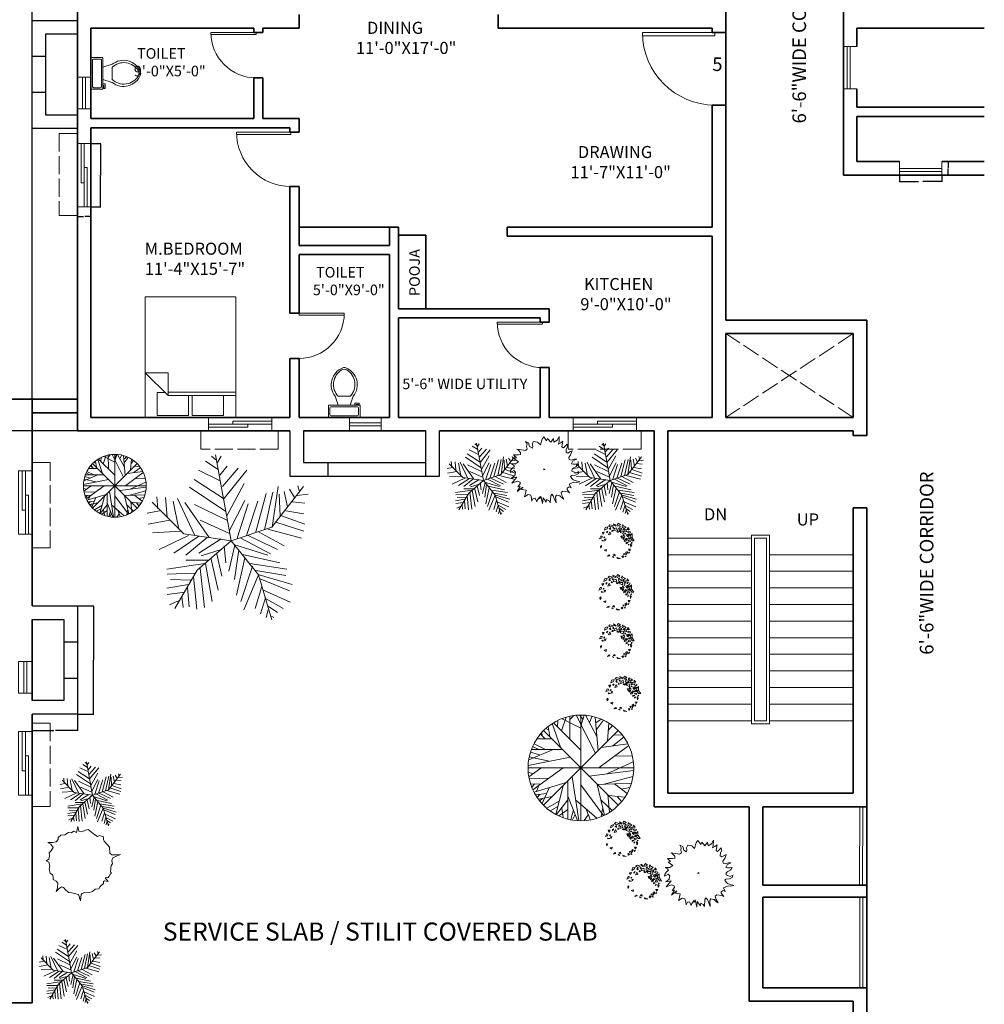
# Model space of a CAD drawing. Units: inches. Extents: x -69 to 2453, y 4803 to 7122.
# Tile 7 of 9: x 1203 to 1843, y 5759 to 6411. Entities that reach past the tile are written whole.
import ezdxf

# ---------------------------------------------------------------- set-up
doc = ezdxf.new("R2010")
doc.units = ezdxf.units.IN
doc.linetypes.add('ACAD_ISO02W100', pattern=[15, 12, -3])
for name, color, linetype, lineweight in [('A-ANNO-DIMS', 2, 'Continuous', 18), ('A-ANNO-IDEN', 2, 'Continuous', 18), ('A-ANNO-TEXT', 7, 'Continuous', 18), ('A-AREA-IDEN', 7, 'Continuous', 18), ('A-DOOR', 3, 'Continuous', 18), ('A-FLOR-FIXT', 9, 'Continuous', 18), ('A-FLOR-OPEN', 8, 'ACAD_ISO02W100', 13), ('A-FLOR-OVHD', 8, 'ACAD_ISO02W100', 13), ('A-FLOR-STRS', 4, 'Continuous', 18), ('A-FURN', 8, 'Continuous', 18), ('A-GLAZ', 244, 'Continuous', 18), ('A-WALL', 7, 'Continuous', 35), ('A-WALL-SRVC', 7, 'Continuous', 30), ('L-PLNT', 94, 'Continuous', 13)]:
    doc.layers.add(name, color=color, linetype=linetype, lineweight=lineweight)
doc.styles.get("Standard").update_dxf_attribs({"font": 'arial.ttf'})
doc.dimstyles.get("Standard").update_dxf_attribs({"dimtxt": 0.18, "dimasz": 0.18, "dimexe": 0.18, "dimexo": 0.0625, "dimgap": 0.09, "dimtad": 0, "dimtih": 1, "dimtoh": 1, "dimdec": 4, "dimzin": 0, "dimdsep": 46, "dimtxsty": 'Standard', "dimcen": 0.09, "dimadec": 0, "dimazin": 0, "dimtfac": 1, "dimtdec": 4, "dimtofl": 0, "dimtmove": 0, "dimatfit": 3, "dimfxl": 1, "dimtolj": 1, "dimtzin": 0, "dimarcsym": 0})

# ---------------------------------------------------------------- blocks, each defined once
blk = doc.blocks.new('*U9')
for p, q in [((0, 0), (0, 6)), ((40, 0), (40, 6))]:
    blk.add_line(p, q)
blk.add_lwpolyline([(0, 0), (0, -40), (1.75, -40), (1.75, 0)], close=True)
blk.add_arc((0, 0), 40, 270, 360)
blk = doc.blocks.new('*U8')
for p, q in [((0, 0), (0, 6)), ((40, 0), (40, 6))]:
    blk.add_line(p, q)
blk.add_lwpolyline([(0, 0), (0, -40), (1.75, -40), (1.75, 0)], close=True)
blk.add_arc((0, 0), 40, 270, 0)
blk = doc.blocks.new('*U5')
for p, q in [((0, 0), (0, -6)), ((40, 0), (40, -6))]:
    blk.add_line(p, q)
blk.add_lwpolyline([(0, 0), (0, 40), (1.75, 40), (1.75, 0)], close=True)
blk.add_arc((0, 0), 40, 0, 90)
blk = doc.blocks.new('*U25')
for p, q in [((-8.737, 47.138), (-17.069, 52.711)), ((-10.186, 53.64), (-13.084, 55.962)), ((0, 0), (-10.5, 57)), ((-9.099, 51.782), (-6.563, 55.962)), ((-7.288, 39.707), (-21.778, 46.673)), ((-7.65, 43.423), (-2.578, 49.46)), ((-5.839, 35.992), (4.667, 48.067)), ((-5.114, 27.632), (10.463, 46.673)), ((-5.114, 28.097), (-24.676, 40.636)), ((-3.665, 19.273), (-27.574, 35.527)), ((-2.941, 16.486), (8.652, 37.85)), ((27, 9), (48, 36)), ((27.127, 9.056), (31.112, 35.992)), ((35.096, 32.741), (37.27, 22.524)), ((38.719, 34.134), (41.979, 28.561)), ((44.153, 36.456), (45.239, 32.741)), ((-48.585, 21.131), (-49.309, 29.026)), ((-43.513, 28.561), (-42.427, 15.558)), ((-38.442, 26.239), (-34.819, 7.663)), ((-35.544, 28.097), (-24.314, 3.947)), ((-1.129, 6.734), (9.014, 26.704)), ((10.101, 3.483), (17.708, 26.239)), ((16.259, 5.805), (23.142, 31.348)), ((22.055, 7.198), (27.489, 32.277)), ((31.836, 30.883), (32.561, 16.486)), ((43.791, 29.954), (51.036, 30.883)), ((-47.498, 19.737), (-55.83, 18.344)), ((-31.5, 4.5), (-52.5, 25.5)), ((-14.533, 2.09), (-30.834, 25.31)), ((-24.314, 23.917), (-2.941, 13.7)), ((3.942, 1.625), (11.187, 24.381)), ((36.183, 19.737), (48.137, 17.88)), ((40.53, 25.775), (48.862, 24.846)), ((-40.615, 13.7), (-55.105, 10.913)), ((-20.691, 13.7), (-1.129, 4.876)), ((33.285, 16.486), (48.862, 10.913)), ((0, 0), (27, 9)), ((24.229, 7.663), (46.688, 1.625)), ((29.662, 12.307), (48.137, 6.269)), ((-33.37, 6.269), (-52.207, 5.34)), ((-28.299, 3.483), (-47.86, -5.805)), ((-21.416, 3.018), (-38.079, -8.128)), ((0, 0), (-31.5, 4.5)), ((-15.982, 2.09), (-30.11, -9.521)), ((0, 0), (-22.5, -19.5)), ((-6.563, 1.161), (-21.416, -8.128)), ((0, 0), (18, -22.5)), ((6.478, 1.625), (26.04, -8.592)), ((11.187, 3.483), (30.749, -5.805)), ((18.07, 5.805), (35.096, -3.483)), ((-6.563, -5.805), (-19.967, -9.985)), ((-4.752, -3.483), (-3.665, -14.629)), ((2.493, -3.019), (-1.491, -20.202)), ((1.769, -2.555), (24.229, -9.521)), ((5.029, -6.27), (2.131, -25.775)), ((-15.257, -12.772), (-30.11, -12.772)), ((-13.446, -11.378), (-8.737, -32.741)), ((-9.461, -8.592), (-6.201, -23.453)), ((9.014, -11.378), (3.58, -35.992)), ((7.565, -9.056), (32.198, -14.629)), ((-17.431, -15.094), (-42.789, -18.809)), ((-22.5, -19.5), (-37.5, -45)), ((-20.691, -18.345), (-17.793, -44.352)), ((-17.069, -15.094), (-12.721, -40.172)), ((14.085, -16.951), (6.478, -40.172)), ((12.274, -15.094), (36.907, -18.809)), ((-24.314, -21.596), (-42.427, -22.06)), ((-26.849, -26.24), (-40.253, -25.775)), ((-25.038, -23.918), (-22.865, -45.281)), ((18.07, -22.524), (8.289, -45.745)), ((16.259, -19.738), (36.183, -22.989)), ((18, -22.5), (27, -52.5)), ((18.433, -22.524), (40.53, -29.026)), ((19.157, -25.311), (38.719, -33.206)), ((-28.299, -29.026), (-42.789, -31.348)), ((-29.023, -30.884), (-27.936, -43.887)), ((20.244, -30.419), (15.897, -44.816)), ((-30.834, -34.135), (-42.427, -35.528)), ((-32.646, -36.921), (-31.921, -44.352)), ((22.78, -37.85), (19.519, -48.532)), ((21.331, -32.741), (39.081, -40.636)), ((22.78, -38.314), (34.372, -44.816)), ((-34.457, -39.708), (-40.978, -42.494)), ((24.591, -43.423), (30.749, -47.603)), ((24.591, -45.745), (23.142, -50.854)), ((26.764, -49.925), (28.213, -50.854))]:
    blk.add_line(p, q)
blk = doc.blocks.new('*U30')
for points in [[(0, 60.64), (-3.051, 56.238), (-4.196, 52.815), (-5.34, 47.925), (-6.103, 45.969), (-11.062, 50.859), (-18.691, 52.326), (-20.98, 47.436), (-20.217, 43.524), (-20.598, 39.611), (-25.939, 43.035), (-27.846, 49.392), (-33.186, 52.326), (-30.516, 47.436), (-31.279, 43.035), (-30.135, 38.144), (-33.568, 35.21), (-40.815, 36.677), (-49.208, 38.144), (-46.919, 36.677), (-42.341, 31.787), (-42.341, 28.364), (-46.537, 27.386), (-55.692, 27.386), (-49.97, 22.006), (-54.548, 21.028), (-46.156, 14.671), (-51.496, 11.248), (-59.888, 11.248), (-55.692, 8.803), (-53.785, 5.38), (-57.218, 3.423), (-60.651, -1.467), (-61.033, -4.89), (-59.125, -3.423), (-54.548, -1.467), (-51.496, -4.401), (-53.022, -10.269), (-59.125, -15.16), (-49.208, -13.204), (-58.362, -24.451), (-48.445, -21.028), (-43.486, -22.495), (-43.104, -25.918), (-47.3, -31.298), (-43.104, -30.32), (-48.445, -39.611), (-38.527, -31.787), (-40.815, -36.188), (-32.423, -37.166), (-33.568, -43.523), (-35.475, -49.392), (-28.609, -44.99), (-23.65, -46.457), (-22.124, -51.837), (-21.743, -57.705), (-19.073, -52.326), (-15.639, -51.837), (-12.588, -58.683), (-11.062, -54.771), (-6.866, -49.392), (-6.866, -53.304), (-4.959, -48.414), (-1.907, -61.617), (-1.144, -51.348), (4.578, -59.172), (5.341, -54.282), (9.918, -56.727), (12.207, -60.639), (12.97, -47.925), (14.877, -44.501), (17.547, -47.436), (19.455, -52.815), (22.888, -60.639), (21.743, -49.392), (23.65, -46.457), (29.754, -47.925), (35.094, -52.326), (37.001, -53.793), (33.187, -46.457), (32.042, -41.567), (35.094, -39.122), (43.868, -40.589), (47.682, -42.056), (43.105, -36.188), (43.105, -33.743), (46.538, -31.298), (50.352, -32.765), (46.919, -26.407), (55.693, -22.495), (60.652, -22.984), (66.374, -22.006), (59.889, -20.05), (54.167, -18.094), (51.878, -15.649), (49.589, -12.225), (51.497, -10.269), (57.981, -9.78), (63.322, -7.335), (64.466, -2.934)], [(64.848, -2.934), (59.507, -5.379), (56.456, -4.401), (51.878, -2.445), (52.26, 0.978), (55.311, 3.912), (59.889, 5.869), (62.94, 11.248), (58.363, 10.27), (54.548, 10.27), (51.115, 11.248), (53.785, 15.649), (57.981, 18.094), (60.652, 19.561), (56.074, 19.561), (51.115, 17.605), (46.538, 19.072), (46.156, 22.496), (49.589, 27.386), (52.26, 34.721), (49.589, 33.743), (44.249, 30.32), (41.197, 32.276), (41.579, 37.655), (43.868, 42.546), (43.105, 46.947), (40.053, 44.013), (36.238, 40.589), (33.568, 42.057), (33.95, 45.969), (35.476, 52.815), (31.28, 49.392), (26.702, 46.947), (28.228, 50.859), (28.609, 61.129), (24.795, 54.282), (18.692, 50.859), (17.929, 57.706), (12.97, 50.859), (7.248, 57.706), (5.341, 53.304), (0, 60.64)]]:
    blk.add_lwpolyline(points)
blk.add_lwpolyline([(0.382, 1.956), (0, 0), (1.907, 0.489), (2.289, 1.467)], close=True)
blk = doc.blocks.new('*U28')
for p, q in [((-22.0458, 42.0753), (-16.5881, 57.6486)), ((-12.5388, 54.9406), (-7.9613, 59.4546)), ((-12.3627, 32.1443), (-12.5388, 58.7776)), ((-5.3205, 59.6806), (16.5105, 16.7963)), ((2.426, 54.9406), (-1.4472, 59.9056)), ((0, 59.9996), (0, -60)), ((0.4894, 48.6208), (3.6584, 59.6806)), ((18.2711, 35.5298), (5.419, 59.6806)), ((9.8203, 51.5549), (12.8133, 58.5516)), ((19.6795, 19.5047), (16.3344, 57.6486)), ((-37.0107, 47.0408), (-35.25, 35.5298)), ((-32.6092, 50.4264), (-23.2782, 23.5674)), ((-31.2008, 51.1035), (-0.2149, 20.1818)), ((-26.4472, 46.5894), (-26.2712, 53.8116)), ((-21.1656, 55.8436), (-0.0388, 45.0094)), ((17.0387, 51.1035), (23.2006, 55.1666)), ((17.7429, 43.6552), (25.4894, 54.2636)), ((31.6513, 50.8778), (30.2429, 30.5643)), ((31.1232, 42.5267), (35.8767, 48.1693)), ((-45.8134, 38.2383), (-40.5318, 33.0471)), ((-43.8768, 36.4326), (-44.405, 40.2696)), ((42, 42), (-42, -42)), ((42, -42), (-42, 42)), ((-40.1797, 44.558), (-36.4825, 43.2038)), ((36.2288, 25.1474), (48.9049, 35.0784)), ((37.1091, 37.1098), (46.6161, 37.5612)), ((-54.7923, 24.4702), (-47.75, 21.0847)), ((-53.2078, 27.4044), (-40.1797, 20.859)), ((-49.8627, 32.8214), (-32.7853, 32.8214)), ((54.3626, 25.3731), (20.9119, 0.3198)), ((23.3767, 23.3417), (53.3063, 27.4044)), ((-59.7219, 2.8025), (-12.0106, 12.0565)), ((-32.2571, 20.6333), (-59.1937, 9.348)), ((-58.6656, 12.7336), (-35.9543, 7.5424)), ((-57.081, 17.9248), (-47.0458, 14.7649)), ((-56.0247, 20.859), (-20.8134, 20.859)), ((38.5175, 13.4107), (58.2359, 13.6364)), ((-54.6162, -24.7335), (-20.2853, 0.0941)), ((29.3626, -6.6771), (59.4682, 7.091)), ((-60, 0), (60, 0)), ((-59.7219, -4.8714), (-54.2641, -6.6771)), ((-45.2853, -0.1316), (-59.0177, -10.0627)), ((-10.074, -10.0627), (-2.5036, -59.7178)), ((9.2922, -9.1598), (59.6443, -2.8401)), ((26.3697, -18.4138), (58.9401, -9.8369)), ((-58.4895, -12.3197), (-36.4825, -11.6426)), ((-57.081, -18.4138), (-45.2853, -17.9624)), ((-52.6797, -18.188), (-55.4966, -22.0251)), ((-53.2078, -27.442), (-16.7641, -16.6081)), ((-47.2219, -19.3166), (-50.2148, -26.3135)), ((-19.9331, -20.2194), (-28.5599, -52.721)), ((-14.8275, -15.0282), (-14.6515, -57.6865)), ((-0.0388, -19.0909), (25.8415, -53.8495)), ((18.6232, -18.6394), (26.7218, -53.3981)), ((18.7992, -18.6394), (57.3556, -17.2853)), ((38.1654, -18.188), (52.426, -29.0219)), ((45.9119, -24.0564), (55.595, -22.2508)), ((-38.9472, -29.0219), (-51.4472, -30.6018)), ((-46.5177, -30.1504), (-49.5106, -33.536)), ((-32.4331, -32.4075), (-48.1021, -35.5674)), ((-35.9543, -22.4765), (-44.0529, -40.5329)), ((-14.6515, -32.1818), (-3.912, -59.4922)), ((30.419, -30.1504), (32.3556, -50.0125)), ((31.4753, -31.279), (49.6091, -33.3103)), ((41.5105, -32.6332), (46.088, -38.0501)), ((-43.7008, -34.6645), (-46.6937, -37.373)), ((-24.6867, -37.8244), (-38.7712, -45.7241)), ((-26.2712, -43.9185), (-34.7219, -48.6583)), ((-14.6515, -36.2445), (-27.6797, -52.9467)), ((-6.2008, -36.2445), (17.919, -57.0094)), ((22.8485, -36.4702), (35.3485, -48.4326)), ((-14.6515, -47.3041), (-25.0388, -54.3009)), ((-21.5177, -45.4984), (-19.9331, -56.1065)), ((-8.4895, -47.5298), (-11.4825, -58.5893)), ((-6.3768, -52.721), (-9.3698, -58.815)), ((8.4119, -53.1724), (3.8344, -59.4922)), ((5.9471, -46.6269), (10.5246, -58.5893)), ((24.7852, -44.8213), (23.0246, -54.978))]:
    blk.add_line(p, q)
blk.add_circle((0, 0), 60)
blk = doc.blocks.new('*U29')
blk.add_lwpolyline([(-4.577, 66.508), (-7.629, 55.26), (-12.588, 57.705), (-17.165, 54.771), (-22.124, 55.26), (-29.372, 50.859), (-36.619, 50.37), (-41.578, 45.968), (-41.578, 42.056), (-45.393, 37.655), (-52.259, 36.677), (-60.651, 36.677), (-54.929, 33.743), (-51.115, 27.385), (-54.548, 21.028), (-58.362, 17.116), (-57.599, 11.248), (-58.744, 5.379), (-63.703, 2.445), (-59.125, 0), (-56.837, -6.846), (-58.362, -13.204), (-56.455, -20.539), (-52.259, -23.473), (-51.115, -27.386), (-51.115, -32.276), (-45.011, -35.21), (-41.96, -39.122), (-42.723, -47.925), (-45.393, -54.282), (-40.434, -49.392), (-35.475, -45.969), (-31.66, -46.947), (-27.083, -51.837), (-21.361, -56.238), (-16.021, -56.727), (-3.433, -60.151), (0, -71.887), (1.526, -60.151), (3.052, -58.194), (8.392, -56.238), (14.114, -56.727), (22.506, -54.282), (27.465, -50.37), (33.95, -49.392), (37.002, -44.991), (42.723, -39.611), (43.105, -35.699), (45.012, -34.721), (51.878, -36.188), (46.157, -29.342), (51.878, -28.364), (53.785, -25.919), (56.074, -21.517), (57.6, -20.539), (55.693, -18.094), (57.219, -5.868), (59.889, -2.934), (58.744, 3.423), (60.27, 7.824), (67.137, 11.248), (74.766, 14.182), (67.899, 13.693), (58.363, 13.693), (54.93, 16.627), (54.167, 27.874), (50.353, 32.276), (43.868, 39.122), (42.723, 42.545), (43.105, 47.436), (35.476, 49.881), (31.661, 47.925), (27.084, 50.859), (14.496, 61.128), (9.155, 59.661), (2.289, 56.727), (-3.051, 57.705)], close=True)
blk = doc.blocks.new('*U27')
for points in [[(-5.78, 9.75), (-7.54, 9.23), (-8.01, 7.5), (-6.26, 8.45)], [(-5.78, 6.81), (-6.66, 6.21), (-6.52, 5.69)], [(-4.43, 11.05), (-5.18, 10.36), (-3.96, 9.49), (-2.07, 10.36)], [(-4.84, 8.63), (-3.83, 7.85), (-4.03, 8.97)], [(-2.88, 7.5), (-3.15, 6.64), (-2.27, 6.72)], [(-1.94, 9.49), (-2.48, 8.97), (-2.27, 8.54), (-1.8, 9.06)], [(-2, 11.66), (-1.6, 10.62), (-0.52, 10.1), (-0.18, 10.62), (-0.79, 10.96)], [(0.02, 9.06), (-1.33, 8.54), (-1.73, 7.16), (0.29, 7.76)], [(0.76, 7.16), (0.09, 6.46), (1.1, 5.95)], [(1.24, 12), (0.56, 11.31), (0.76, 10.01), (2.52, 11.05)], [(1.37, 8.54), (3.13, 8.8), (3.8, 7.85), (1.91, 7.76)], [(2.59, 9.93), (1.84, 9.75), (1.64, 9.23), (2.32, 9.41)], [(1.71, 6.29), (1.71, 7.07), (2.65, 7.5), (2.11, 6.9)], [(2.52, 6.81), (2.52, 5.86), (4.41, 5.17), (4.61, 6.72)], [(4.14, 11.14), (3.6, 10.01), (4, 9.23), (5.22, 8.71), (6.3, 9.41), (5.08, 10.19), (4.61, 10.01)], [(4.61, 8.28), (4.54, 7.76), (4.95, 7.59), (4.95, 8.28)], [(6.43, 7.94), (5.49, 7.68), (5.56, 6.21), (6.5, 6.64)], [(7.45, 9.32), (7.11, 7.94), (8.52, 7.94)], [(7.85, 6.81), (7.18, 6.21), (9, 5.51), (9.33, 6.38)], [(-11.32, 1.79), (-9.83, 2.31), (-9.63, 3.44), (-10.44, 3.52)], [(-8.21, 0.41), (-9.43, 0.32), (-9.83, 0.84)], [(-8.14, 6.03), (-9.36, 5.95), (-9.02, 4.73)], [(-8.21, 3.09), (-8.48, 2.31), (-7.87, 2.57)], [(-7, 1.79), (-7.94, 1.53), (-7.47, 0.49)], [(-4.57, 6.38), (-5.45, 4.47), (-3.89, 4.82)], [(3.53, 1.88), (2.86, 3.52), (3.8, 3.52)], [(4.41, 4.56), (4.27, 3.7), (5.49, 3.26)], [(4.27, 2.74), (5.29, 2.66), (4.41, 1.27)], [(5.83, 1.53), (5.02, 0.41), (5.49, -0.02), (6.5, 0.41)], [(5.49, 5.51), (5.42, 4.82), (6.16, 5.08)], [(7.51, 1.71), (6.91, 1.27), (6.23, 2.14)], [(8.12, 4.99), (7.11, 4.65), (6.5, 4.13), (7.38, 3.09), (8.12, 3.52), (7.65, 3.87)], [(8.12, 0.75), (7.51, 0.15), (8.93, -0.28), (9.13, 0.49)], [(8.19, 2.57), (7.92, 2.05), (8.66, 1.53)], [(8.73, 4.73), (8.19, 4.56), (8.39, 3.87), (8.59, 4.04)], [(10.28, 5.17), (9.2, 4.04), (9, 2.31), (10.48, 0.49), (11.76, 0.41), (10.35, 2.48), (9.33, 2.4), (10.28, 2.83)], [(-10.03, -2.71), (-10.64, -3.31), (-10.44, -4.44), (-9.9, -3.49)], [(-8.28, -5.73), (-6.79, -5.3), (-7, -6.51)], [(7.78, -0.8), (6.43, -1.5), (6.43, -0.72)], [(8.32, -1.75), (7.98, -2.53), (7.58, -2.1)], [(9.33, -5.13), (8.46, -6.25), (7.98, -5.22)], [(9.33, -1.75), (9.54, -3.74), (10.14, -2.53)], [(10.08, -0.63), (9.74, -1.32), (10.48, -0.89)], [(-4.84, -8.85), (-4.43, -9.45), (-5.99, -9.8)], [(-2.54, -10.06), (-3.02, -10.23), (-1.8, -10.67)], [(-2.34, -9.2), (-1.26, -8.5), (-0.99, -9.54)], [(0.22, -10.58), (0.83, -11.27), (2.59, -11.36)], [(4.07, -9.45), (3.53, -9.97), (4.07, -10.58), (4.61, -9.89)], [(5.29, -7.98), (4.61, -8.16), (5.02, -8.94)], [(6.03, -9.45), (5.42, -9.97), (6.16, -10.15)], [(6.1, -8.94), (6.16, -7.21), (6.91, -6.69), (7.24, -7.38)], [(8.05, -8.07), (8.59, -7.12), (7.92, -7.55)]]:
    blk.add_lwpolyline(points, close=True)
blk = doc.blocks.new('Bed - Queen')
for p, q in [((0, -80.00003), (0, 0)), ((0, 0), (59.99999, 0)), ((59.99999, 0), (59.99999, -80.00003)), ((7.99999, -1.2), (28.79998, -1.2)), ((7.99999, -14.4), (7.99999, -1.2)), ((28.79998, -1.2), (28.79998, -14.4)), ((31.19999, -1.2), (51.99999, -1.2)), ((31.19999, -14.4), (31.19999, -1.2)), ((51.99999, -1.2), (51.99999, -16.4)), ((0, -14.4), (44.8, -14.4)), ((44.8, -16.8), (0, -16.8)), ((59.99999, -29.6), (44.8, -14.4)), ((44.8, -14.4), (44.8, -29.6)), ((51.99999, -16.4), (46.79936, -16.4)), ((44.8, -29.6), (59.99999, -29.6)), ((59.99999, -80.00003), (0, -80.00003))]:
    blk.add_line(p, q)
blk = doc.blocks.new('*U33')
for p, q in [((9.5, -6), (9.5, -2)), ((-10, -8.5), (-8, -8.5)), ((-10, -9.5), (-10, -8.5)), ((-7, -9.5), (-10, -9.5)), ((-8, -8.5), (-8, -8)), ((-7, -8), (-7, -9.5)), ((-4, -8), (-6, -14)), ((4, -8), (6, -14)), ((4, -14), (-4, -14))]:
    blk.add_line(p, q)
blk.add_lwpolyline([(10.5, -8), (10.5, 0), (-10.5, 0), (-10.5, -8)], close=True)
for points in [[(-9.5, -2), (-9.5, -6)], [(8.5, -1), (-8.5, -1)], [(-8.5, -7), (8.5, -7)]]:
    blk.add_lwpolyline(points)
for centre, radius, start, end in [((-8.62, -1.88), 0.884, 81.8699, 188.1301), ((-8.62, -6.12), 0.884, 171.8699, 278.1301), ((8.62, -1.88), 0.884, 351.8699, 98.1301), ((8.62, -6.12), 0.884, 261.8699, 8.1301), ((3.52, -21.58), 12.17, 141.46911, 247.97143), ((4.2, -21.82), 11.33, 136.36773, 238.94682), ((-3.52, -21.58), 12.17, 292.02843, 38.53071), ((-4.2, -21.82), 11.33, 301.05301, 43.63209), ((0, -27.88), 4, 245.73182, 294.26817), ((0, -29), 4, 254.86053, 285.13947)]:
    blk.add_arc(centre, radius, start, end)
blk = doc.blocks.new('WINDOW-VENT-21IN')
for p, q in [((0, 5.5), (21, 5.5)), ((0, 3.5), (21, 3.5))]:
    blk.add_line(p, q)
blk.add_lwpolyline([(0, 9), (21, 9), (21, 0), (0, 0)], close=True)
blk = doc.blocks.new('WINDOW-SLIDING-42IN')
for p, q in [((2.5, 42), (2.5, 16)), ((4.5, 42), (4.5, 0)), ((4.5, 26), (6.5, 26)), ((6.5, 26), (6.5, 0)), ((4.5, 16), (2.5, 16))]:
    blk.add_line(p, q)
blk.add_lwpolyline([(0, 42), (9, 42), (9, 0), (0, 0)], close=True)
blk = doc.blocks.new('SUNSHADE-54IN')
for p, q in [((12, 54.34), (0, 54.34)), ((0, 54.34), (0, 0)), ((0, 0), (12, 0))]:
    blk.add_line(p, q)
blk = doc.blocks.new('SUNSHADE-48IN')
for p, q in [((0, 0), (0, 12)), ((48.4, 12), (48.4, 0)), ((48.4, 0), (0, 0))]:
    blk.add_line(p, q)
blk = doc.blocks.new('SERVICE-BAY-99IN')
for p, q in [((0, 30), (0, 0)), ((9, 30), (9, 9)), ((90.11, 0), (90.11, 30)), ((99.11, 0), (99.11, 30)), ((9, 9), (90.11, 9)), ((25.44, 0), (25.44, 9)), ((0, 0), (99.11, 0))]:
    blk.add_line(p, q)
blk = doc.blocks.new('SERVICE-BAY-72IN')
for p, q in [((0, 71.78), (30, 71.78)), ((30, 71.78), (30, 0)), ((0, 62.78), (21, 62.78)), ((21, 62.78), (21, 9)), ((21, 47.89), (30, 47.89)), ((21, 23.89), (30, 23.89)), ((21, 9), (0, 9)), ((30, 0), (0, 0))]:
    blk.add_line(p, q)
blk = doc.blocks.new('WINDOW-CORE-28IN')
for p, q in [((0, 9), (0, 0)), ((28, 9), (28, 0)), ((28, 4.5), (0, 4.5)), ((28, 2.5), (0, 2.5))]:
    blk.add_line(p, q)
blk = doc.blocks.new('*D49')
at = {"layer": 'A-ANNO-DIMS', "color": 0, "lineweight": -2, "transparency": 16777216}
for p, q in [((1250.57, 6329.26), (1256.99, 6329.26)), ((1256.81, 6329.08), (1256.81, 6308.45)), ((1256.81, 6287.44), (1256.81, 6308.08)), ((1250.57, 6287.26), (1256.99, 6287.26))]:
    blk.add_line(p, q, dxfattribs=at)
at = {"layer": 'A-ANNO-DIMS', "color": 0, "transparency": 16777216}
for points in [[(1256.78, 6329.08), (1256.84, 6329.08), (1256.81, 6329.26)], [(1256.78, 6287.44), (1256.84, 6287.44), (1256.81, 6287.26)]]:
    blk.add_solid(points, dxfattribs=at)
at = {"layer": 'Defpoints', "color": 0, "transparency": 16777216}
for p in [(1250.51, 6329.26), (1256.81, 6329.26), (1250.51, 6287.26)]:
    blk.add_point(p, dxfattribs=at)
at = {"layer": 'A-ANNO-DIMS', "color": 0, "transparency": 16777216, "insert": (1256.81, 6308.26), "char_height": 0.18, "attachment_point": 5}
blk.add_mtext('\\A1;SLIDING WINDOW 42 TYP.', dxfattribs=at)
blk = doc.blocks.new('*D50')
at = {"layer": 'A-ANNO-DIMS', "color": 0, "lineweight": -2, "transparency": 16777216}
for p, q in [((1241.51, 6287.2), (1241.51, 6280.78)), ((1250.51, 6287.2), (1250.51, 6280.78)), ((1241.69, 6280.96), (1245.55, 6280.96)), ((1250.33, 6280.96), (1246.47, 6280.96))]:
    blk.add_line(p, q, dxfattribs=at)
at = {"layer": 'A-ANNO-DIMS', "color": 0, "transparency": 16777216}
for points in [[(1241.69, 6280.99), (1241.69, 6280.93), (1241.51, 6280.96)], [(1250.33, 6280.99), (1250.33, 6280.93), (1250.51, 6280.96)]]:
    blk.add_solid(points, dxfattribs=at)
at = {"layer": 'Defpoints', "color": 0, "transparency": 16777216}
for p in [(1241.51, 6287.26), (1250.51, 6287.26), (1250.51, 6280.96)]:
    blk.add_point(p, dxfattribs=at)
at = {"layer": 'A-ANNO-DIMS', "color": 0, "transparency": 16777216, "insert": (1246.01, 6280.96), "char_height": 0.18, "attachment_point": 5}
blk.add_mtext('\\A1;9 TYP.', dxfattribs=at)
blk = doc.blocks.new('*D75')
at = {"layer": 'A-ANNO-DIMS', "color": 0, "lineweight": -2, "transparency": 16777216}
for p, q in [((1241.57, 6022.79), (1252.46, 6022.79)), ((1252.28, 6022.61), (1252.28, 5987.08)), ((1252.28, 5951.19), (1252.28, 5986.72)), ((1241.57, 5951.01), (1252.46, 5951.01))]:
    blk.add_line(p, q, dxfattribs=at)
at = {"layer": 'A-ANNO-DIMS', "color": 0, "transparency": 16777216}
for points in [[(1252.25, 6022.61), (1252.31, 6022.61), (1252.28, 6022.79)], [(1252.25, 5951.19), (1252.31, 5951.19), (1252.28, 5951.01)]]:
    blk.add_solid(points, dxfattribs=at)
at = {"layer": 'Defpoints', "color": 0, "transparency": 16777216}
for p in [(1241.51, 6022.79), (1252.28, 6022.79), (1241.51, 5951.01)]:
    blk.add_point(p, dxfattribs=at)
at = {"layer": 'A-ANNO-DIMS', "color": 0, "transparency": 16777216, "insert": (1252.28, 5986.9), "char_height": 0.18, "attachment_point": 5}
blk.add_mtext('\\A1;SERVICE BAY 72 TYP.', dxfattribs=at)
blk = doc.blocks.new('*D76')
at = {"layer": 'A-ANNO-DIMS', "color": 0, "lineweight": -2, "transparency": 16777216}
for p, q in [((1211.51, 5950.95), (1211.51, 5940.07)), ((1241.51, 5950.95), (1241.51, 5940.07)), ((1211.69, 5940.25), (1225.98, 5940.25)), ((1241.33, 5940.25), (1227.04, 5940.25))]:
    blk.add_line(p, q, dxfattribs=at)
at = {"layer": 'A-ANNO-DIMS', "color": 0, "transparency": 16777216}
for points in [[(1211.69, 5940.28), (1211.69, 5940.22), (1211.51, 5940.25)], [(1241.33, 5940.28), (1241.33, 5940.22), (1241.51, 5940.25)]]:
    blk.add_solid(points, dxfattribs=at)
at = {"layer": 'Defpoints', "color": 0, "transparency": 16777216}
for p in [(1211.51, 5951.01), (1241.51, 5951.01), (1241.51, 5940.25)]:
    blk.add_point(p, dxfattribs=at)
at = {"layer": 'A-ANNO-DIMS', "color": 0, "transparency": 16777216, "insert": (1226.51, 5940.25), "char_height": 0.18, "attachment_point": 5}
blk.add_mtext('\\A1;30 TYP.', dxfattribs=at)
blk = doc.blocks.new('*D79')
at = {"layer": 'A-ANNO-DIMS', "color": 0, "lineweight": -2, "transparency": 16777216}
for p, q in [((1786.76, 6308.15), (1786.76, 6303.84)), ((1786.94, 6304.02), (1799.25, 6304.02)), ((1814.58, 6304.02), (1802.27, 6304.02)), ((1814.76, 6308.15), (1814.76, 6303.84))]:
    blk.add_line(p, q, dxfattribs=at)
at = {"layer": 'A-ANNO-DIMS', "color": 0, "transparency": 16777216}
for points in [[(1786.94, 6304.05), (1786.94, 6303.99), (1786.76, 6304.02)], [(1814.58, 6304.05), (1814.58, 6303.99), (1814.76, 6304.02)]]:
    blk.add_solid(points, dxfattribs=at)
at = {"layer": 'Defpoints', "color": 0, "transparency": 16777216}
for p in [(1786.76, 6308.22), (1814.76, 6308.22), (1814.76, 6304.02)]:
    blk.add_point(p, dxfattribs=at)
at = {"layer": 'A-ANNO-DIMS', "color": 0, "transparency": 16777216, "insert": (1800.76, 6304.02), "char_height": 0.18, "attachment_point": 5}
blk.add_mtext('\\A1;CORE WINDOW 28 TYP.', dxfattribs=at)
blk = doc.blocks.new('*D80')
at = {"layer": 'A-ANNO-DIMS', "color": 0, "lineweight": -2, "transparency": 16777216}
for p, q in [((1814.82, 6317.22), (1819.14, 6317.22)), ((1818.96, 6317.04), (1818.96, 6312.9)), ((1818.96, 6308.4), (1818.96, 6312.53)), ((1814.82, 6308.22), (1819.14, 6308.22))]:
    blk.add_line(p, q, dxfattribs=at)
at = {"layer": 'A-ANNO-DIMS', "color": 0, "transparency": 16777216}
for points in [[(1818.93, 6317.04), (1818.99, 6317.04), (1818.96, 6317.22)], [(1818.93, 6308.4), (1818.99, 6308.4), (1818.96, 6308.22)]]:
    blk.add_solid(points, dxfattribs=at)
at = {"layer": 'Defpoints', "color": 0, "transparency": 16777216}
for p in [(1814.76, 6317.22), (1818.96, 6317.22), (1814.76, 6308.22)]:
    blk.add_point(p, dxfattribs=at)
at = {"layer": 'A-ANNO-DIMS', "color": 0, "transparency": 16777216, "insert": (1818.96, 6312.72), "char_height": 0.18, "attachment_point": 5}
blk.add_mtext('\\A1;9 TYP.', dxfattribs=at)
blk = doc.blocks.new('*D100')
at = {"layer": 'A-ANNO-DIMS', "color": 0, "lineweight": -2, "transparency": 16777216}
for p, q in [((752.51, 6159.78), (752.51, 7121.65)), ((752.69, 7121.47), (981.72, 7121.47)), ((1211.33, 7121.47), (982.3, 7121.47)), ((1211.51, 6159.78), (1211.51, 7121.65))]:
    blk.add_line(p, q, dxfattribs=at)
at = {"layer": 'A-ANNO-DIMS', "color": 0, "transparency": 16777216}
for points in [[(752.69, 7121.5), (752.69, 7121.44), (752.51, 7121.47)], [(1211.33, 7121.5), (1211.33, 7121.44), (1211.51, 7121.47)]]:
    blk.add_solid(points, dxfattribs=at)
at = {"layer": 'Defpoints', "color": 0, "transparency": 16777216}
for p in [(1211.51, 7121.47), (752.51, 6159.72), (1211.51, 6159.72)]:
    blk.add_point(p, dxfattribs=at)
at = {"layer": 'A-ANNO-DIMS', "color": 0, "transparency": 16777216, "insert": (982.01, 7121.47), "char_height": 0.18, "attachment_point": 5}
blk.add_mtext('\\A1;459', dxfattribs=at)
blk = doc.blocks.new('*D103')
at = {"layer": 'A-ANNO-DIMS', "color": 0, "lineweight": -2, "transparency": 16777216}
for p, q in [((1241.45, 6552.72), (-69.42, 6552.72)), ((-69.24, 6552.54), (-69.24, 6345.9)), ((-69.24, 6138.9), (-69.24, 6345.53)), ((1241.45, 6138.72), (-69.42, 6138.72))]:
    blk.add_line(p, q, dxfattribs=at)
at = {"layer": 'A-ANNO-DIMS', "color": 0, "transparency": 16777216}
for points in [[(-69.27, 6552.54), (-69.21, 6552.54), (-69.24, 6552.72)], [(-69.27, 6138.9), (-69.21, 6138.9), (-69.24, 6138.72)]]:
    blk.add_solid(points, dxfattribs=at)
at = {"layer": 'Defpoints', "color": 0, "transparency": 16777216}
for p in [(-69.24, 6552.72), (1241.51, 6552.72), (1241.51, 6138.72)]:
    blk.add_point(p, dxfattribs=at)
at = {"layer": 'A-ANNO-DIMS', "color": 0, "transparency": 16777216, "insert": (-69.24, 6345.72), "char_height": 0.18, "attachment_point": 5}
blk.add_mtext('\\A1;414', dxfattribs=at)

msp = doc.modelspace()

# ---------------------------------------------------------------- linework, layer by layer
at = {"layer": 'A-FLOR-OPEN'}
for p, q in [((1756.01, 6203.22), (1671.51, 6147.72)), ((1756.01, 6147.72), (1671.51, 6203.22))]:
    msp.add_line(p, q, dxfattribs=at)
at = {"layer": 'A-FLOR-OVHD'}
for p, q in [((1323.36, 6126.72), (1323.36, 6138.72)), ((1374.62, 6138.72), (1374.62, 6126.72)), ((1374.62, 6126.72), (1323.36, 6126.72)), ((1211.51, 6117.72), (1223.51, 6117.72)), ((1223.51, 6117.72), (1223.51, 6061.25)), ((1223.51, 6061.25), (1211.51, 6061.25)), ((1211.51, 5945.08), (1223.51, 5945.08)), ((1223.51, 5945.08), (1223.51, 5889.88)), ((1223.51, 5889.88), (1211.51, 5889.88))]:
    msp.add_line(p, q, dxfattribs=at)
at = {"layer": 'A-FLOR-STRS'}
for p, q in [((1688.51, 5944.72), (1688.51, 6069.72)), ((1688.51, 6069.72), (1700.51, 6069.72)), ((1700.51, 5944.72), (1700.51, 6069.72)), ((1633.01, 6067.72), (1688.51, 6067.72)), ((1690.51, 5946.72), (1690.51, 6067.72)), ((1690.51, 6067.72), (1698.51, 6067.72)), ((1698.51, 5946.72), (1698.51, 6067.72)), ((1633.01, 6056.72), (1688.51, 6056.72)), ((1700.51, 6056.72), (1756.01, 6056.72)), ((1633.01, 6045.72), (1688.51, 6045.72)), ((1700.51, 6045.72), (1756.01, 6045.72)), ((1633.01, 6034.72), (1688.51, 6034.72)), ((1700.51, 6034.72), (1756.01, 6034.72)), ((1633.01, 6023.72), (1688.51, 6023.72)), ((1700.51, 6023.72), (1756.01, 6023.72)), ((1633.01, 6012.72), (1688.51, 6012.72)), ((1700.51, 6012.72), (1756.01, 6012.72)), ((1633.01, 6001.72), (1688.51, 6001.72)), ((1700.51, 6001.72), (1756.01, 6001.72)), ((1633.01, 5990.72), (1688.51, 5990.72)), ((1700.51, 5990.72), (1756.01, 5990.72)), ((1633.01, 5979.72), (1688.51, 5979.72)), ((1700.51, 5979.72), (1756.01, 5979.72)), ((1633.01, 5968.72), (1688.51, 5968.72)), ((1700.51, 5968.72), (1756.01, 5968.72)), ((1633.01, 5957.72), (1688.51, 5957.72)), ((1700.51, 5957.72), (1756.01, 5957.72)), ((1633.01, 5946.72), (1688.51, 5946.72)), ((1688.51, 5944.72), (1700.51, 5944.72)), ((1690.51, 5946.72), (1698.51, 5946.72)), ((1700.51, 5946.72), (1756.01, 5946.72))]:
    msp.add_line(p, q, dxfattribs=at)
at = {"layer": 'A-GLAZ'}
for p, q in [((1760.16, 5837.72), (1760.51, 5889.72)), ((1762.16, 5837.7), (1762.51, 5889.7)), ((1760.51, 5769.72), (1760.51, 5829.72)), ((1762.51, 5769.72), (1762.51, 5829.72))]:
    msp.add_line(p, q, dxfattribs=at)
at = {"layer": 'A-WALL'}
for p, q in [((1671.51, 6212.22), (1671.51, 6813.72)), ((1749.51, 6308.22), (1749.51, 6813.72)), ((1241.51, 6138.72), (1241.51, 6552.72)), ((1388.51, 6405.72), (1388.51, 6414.72)), ((1520.51, 6405.72), (1520.51, 6414.72)), ((1250.51, 6405.72), (1358.51, 6405.72)), ((1250.51, 6345.72), (1250.51, 6405.72)), ((1358.51, 6402.72), (1358.51, 6405.72)), ((1364.51, 6402.72), (1358.51, 6402.72)), ((1364.51, 6405.72), (1388.51, 6405.72)), ((1364.51, 6402.72), (1364.51, 6405.72)), ((1520.51, 6405.72), (1662.51, 6405.72)), ((1662.51, 6402.72), (1662.51, 6405.72)), ((1662.51, 6402.72), (1671.51, 6402.72)), ((1758.51, 6405.72), (1843.01, 6405.72)), ((1758.51, 6393.47), (1758.51, 6405.72)), ((1358.51, 6345.72), (1358.51, 6372.72)), ((1364.51, 6372.72), (1358.51, 6372.72)), ((1364.51, 6345.72), (1364.51, 6372.72)), ((1758.51, 6353.22), (1758.51, 6365.47)), ((1662.51, 6273.72), (1662.51, 6354.72)), ((1662.51, 6354.72), (1671.51, 6354.72)), ((1758.51, 6353.22), (1843.01, 6353.22)), ((1250.51, 6345.72), (1358.51, 6345.72)), ((1364.51, 6345.72), (1388.51, 6345.72)), ((1388.51, 6336.72), (1388.51, 6345.72)), ((1758.51, 6317.22), (1758.51, 6347.22)), ((1758.51, 6347.22), (1843.01, 6347.22)), ((1250.51, 6147.72), (1250.51, 6339.72)), ((1250.51, 6339.72), (1382.51, 6339.72)), ((1382.51, 6336.72), (1382.51, 6339.72)), ((1382.51, 6336.72), (1388.51, 6336.72)), ((1758.51, 6317.22), (1786.76, 6317.22)), ((1814.76, 6317.22), (1843.01, 6317.22)), ((1749.51, 6308.22), (1843.01, 6308.22)), ((1382.51, 6300.72), (1388.51, 6300.72)), ((1382.51, 6216.72), (1382.51, 6300.72)), ((1388.51, 6261.72), (1388.51, 6300.72)), ((1388.51, 6273.72), (1454.51, 6273.72)), ((1448.51, 6261.72), (1448.51, 6273.72)), ((1454.51, 6219.72), (1454.51, 6273.72)), ((1526.51, 6273.72), (1526.51, 6267.72)), ((1526.51, 6273.72), (1662.51, 6273.72)), ((1454.51, 6268.53), (1472.51, 6268.53)), ((1472.51, 6219.72), (1472.51, 6268.53)), ((1526.51, 6267.72), (1662.51, 6267.72)), ((1662.51, 6147.72), (1662.51, 6267.72)), ((1388.51, 6261.72), (1448.51, 6261.72)), ((1388.51, 6255.72), (1448.51, 6255.72)), ((1388.51, 6216.72), (1388.51, 6255.72)), ((1448.51, 6147.72), (1448.51, 6255.72)), ((1454.51, 6219.72), (1554.51, 6219.72)), ((1554.51, 6210.72), (1554.51, 6219.72)), ((1388.51, 6216.72), (1382.51, 6216.72)), ((1454.51, 6147.72), (1454.51, 6213.72)), ((1454.51, 6213.72), (1548.51, 6213.72)), ((1548.51, 6210.72), (1548.51, 6213.72)), ((1671.51, 6212.22), (1765.01, 6212.22)), ((1765.01, 6212.22), (1765.01, 6135.72)), ((1548.51, 6210.72), (1554.51, 6210.72)), ((1671.51, 6147.72), (1671.51, 6203.22)), ((1671.51, 6203.22), (1756.01, 6203.22)), ((1756.01, 6203.22), (1756.01, 6147.72)), ((1382.51, 6147.72), (1382.51, 6186.72)), ((1388.51, 6186.72), (1382.51, 6186.72)), ((1388.51, 6147.72), (1388.51, 6186.72)), ((1548.51, 6147.72), (1548.51, 6180.72)), ((1548.51, 6180.72), (1554.51, 6180.72)), ((1554.51, 6147.72), (1554.51, 6180.72)), ((752.51, 6159.72), (1241.51, 6159.72)), ((1211.51, 6159.72), (1211.51, 6022.79)), ((1211.51, 6150.72), (1241.51, 6150.72)), ((1250.51, 6147.72), (1382.51, 6147.72)), ((1388.51, 6147.72), (1448.51, 6147.72)), ((1454.51, 6147.72), (1548.51, 6147.72)), ((1554.51, 6147.72), (1662.51, 6147.72)), ((1671.51, 6147.72), (1756.01, 6147.72)), ((1241.51, 6138.72), (1382.51, 6138.72)), ((1391.51, 6138.72), (1472.62, 6138.72)), ((1481.62, 6138.72), (1624.01, 6138.72)), ((1624.01, 6138.72), (1624.01, 5889.72)), ((1633.01, 6138.72), (1633.01, 5898.72)), ((1633.01, 6138.72), (1756.01, 6138.72)), ((1756.01, 6138.72), (1756.01, 6135.72)), ((1756.01, 6135.72), (1765.01, 6135.72)), ((1756.01, 6087.72), (1765.01, 6087.72)), ((1756.01, 6087.72), (1756.01, 5898.72)), ((1765.01, 6087.72), (1765.01, 5466.72)), ((1211.51, 6013.79), (1211.51, 5960.01)), ((1211.51, 5951.01), (1211.51, 5759.72)), ((1633.01, 5898.72), (1756.01, 5898.72)), ((1624.01, 5889.72), (1687.01, 5889.72)), ((1687.01, 5889.72), (1687.01, 5760.72)), ((1696.01, 5889.72), (1696.01, 5837.72)), ((1696.01, 5889.72), (1765.01, 5889.72)), ((1696.01, 5837.72), (1765.01, 5837.72)), ((1696.01, 5829.72), (1765.01, 5829.72)), ((1696.01, 5829.72), (1696.01, 5769.72)), ((1696.01, 5769.72), (1765.01, 5769.72)), ((971.78, 5759.72), (1211.51, 5759.72)), ((1687.01, 5760.72), (1756.01, 5760.72)), ((1756.01, 5760.72), (1756.01, 5475.72))]:
    msp.add_line(p, q, dxfattribs=at)

# ---------------------------------------------------------------- block references
at = {"layer": 'A-DOOR'}
for name, p, xscale, yscale, zscale, rotation in [('*U8', (1360.01, 6402.72), 0.75, 0.75, 0.75, 270.0000000000001), ('*U9', (1664.31, 6402.72), 1.199999999999977, 1.199999999999977, 1.199999999999977, 270.0000000000001), ('*U8', (1383.11, 6336.72), 0.9, 0.9, 0.9, 270), ('*U5', (1388.51, 6216.72), 0.75, 0.75, 0.75, 270.0000000000001), ('*U8', (1550.01, 6210.72), 0.75, 0.75, 0.75, 270.0000000000001)]:
    msp.add_blockref(name, p, dxfattribs=dict(at, xscale=xscale, yscale=yscale, zscale=zscale, rotation=rotation))
at = {"layer": 'A-FLOR-FIXT'}
for p, rotation in [((1250.51, 6375.72), 89.99999999999999), ((1418.51, 6147.72), 180)]:
    msp.add_blockref('*U33', p, dxfattribs=dict(at, rotation=rotation))
at = {"layer": 'A-FLOR-OVHD'}
for name, p in [('SUNSHADE-54IN', (1229.51, 6281.61)), ('SUNSHADE-48IN', (1566.92, 6126.72))]:
    msp.add_blockref(name, p, dxfattribs=at)
at = {"layer": 'A-FURN', "rotation": 180}
msp.add_blockref('Bed - Queen', (1346.51, 6147.72), dxfattribs=at)
at = {"layer": 'A-GLAZ'}
for name, p, rotation in [('WINDOW-CORE-28IN', (1749.51, 6393.47), 270.0000000000003), ('WINDOW-VENT-21IN', (1241.51, 6373.21), 269.999999999998), ('WINDOW-SLIDING-42IN', (1328.53, 6147.72), 270.000000000003), ('WINDOW-SLIDING-42IN', (1570.38, 6147.72), 269.999999999994), ('WINDOW-VENT-21IN', (1202.51, 5985.87), 269.999999999998)]:
    msp.add_blockref(name, p, dxfattribs=dict(at, rotation=rotation))
for name, p in [('WINDOW-SLIDING-42IN', (1241.51, 6287.26)), ('WINDOW-CORE-28IN', (1786.76, 6308.22)), ('WINDOW-VENT-21IN', (1422.08, 6138.72)), ('WINDOW-SLIDING-42IN', (1202.51, 6070.25)), ('WINDOW-SLIDING-42IN', (1202.51, 5897.44))]:
    msp.add_blockref(name, p, dxfattribs=at)
at = {"layer": 'A-WALL-SRVC', "rotation": 180}
msp.add_blockref('SERVICE-BAY-72IN', (1241.51, 6410.86), dxfattribs=at)
at = {"layer": 'A-WALL-SRVC'}
for name, p in [('SERVICE-BAY-99IN', (1382.51, 6108.72)), ('SERVICE-BAY-72IN', (1211.51, 5951.01))]:
    msp.add_blockref(name, p, dxfattribs=at)
at = {"layer": 'L-PLNT'}
for name, p, xscale, yscale, zscale in [('*U30', (1550.77, 6112.96), 0.3609947042258796, 0.3609947042258796, 0.3609947042258796), ('*U25', (1510.79, 6105.98), 0.4317744748014456, 0.4317744748014456, 0.4317744748014456), ('*U25', (1594.91, 6105.97), 0.4317744748014456, 0.4317744748014456, 0.4317744748014456), ('*U28', (1266.35, 6102.37), 0.3475477793313044, 0.3475477793313044, 0.3475477793313044), ('*U28', (1575.45, 5915.4), 0.5842112454010082, 0.5842112454010082, 0.5842112454010082), ('*U25', (1251.64, 5897.38), 0.3868695086522477, 0.3868695086522477, 0.3868695086522477), ('*U29', (1243.56, 5852.93), 0.356051830328967, 0.356051830328967, 0.356051830328967), ('*U30', (1653.03, 5845.43), 0.3609947042258796, 0.3609947042258796, 0.3609947042258796), ('*U25', (1237.71, 5779.64), 0.3868695086522477, 0.3868695086522477, 0.3868695086522477)]:
    msp.add_blockref(name, p, dxfattribs=dict(at, xscale=xscale, yscale=yscale, zscale=zscale))
for name, p in [('*U25', (1343.55, 6065.97)), ('*U27', (1599.13, 6065.52)), ('*U27', (1598.73, 6031.49)), ('*U27', (1599.13, 5999.15)), ('*U27', (1603.39, 5964.27)), ('*U27', (1602.99, 5868.12)), ('*U27', (1617.16, 5839.98))]:
    msp.add_blockref(name, p, dxfattribs=at)

# ---------------------------------------------------------------- texts
at = {"layer": 'A-ANNO-IDEN', "insert": (1662.57, 6386.27), "char_height": 8, "attachment_point": 1}
msp.add_mtext_dynamic_manual_height_columns('{\\H1.125x;5} ', width=10.4994, gutter_width=12.5, heights=[0], dxfattribs=at)
at = {"layer": 'A-ANNO-TEXT', "char_height": 8, "attachment_point": 1}
for s, insert in [('DN ', (1657.08, 6087.52)), ('UP', (1718.61, 6084.08))]:
    msp.add_mtext_dynamic_manual_height_columns(s, width=16.1756, gutter_width=12.5, heights=[0], dxfattribs=dict(at, insert=insert))
at = {"layer": 'A-AREA-IDEN', "attachment_point": 1, "rotation": 90}
for s, width, insert, char_height in [('6\'-6"WIDE CORRIDOR', 131.0566, (1715.76, 6342.51), 9), ('POOJA', 33.9191, (1461.62, 6228.15), 7), ('6\'-6"WIDE CORRIDOR', 131.0566, (1800.26, 5990.43), 9)]:
    msp.add_mtext_dynamic_manual_height_columns(s, width=width, gutter_width=12.5, heights=[0], dxfattribs=dict(at, insert=insert, char_height=char_height))
at = {"layer": 'A-AREA-IDEN', "attachment_point": 1}
for s, width, insert, char_height in [('   DINING\\P11\'-0"X17\'-0"', 63.2359, (1426.27, 6409.9), 8), (' TOILET\\P9\'-0"X5\'-0"', 45.2514, (1278.97, 6392.42), 7), ('  DRAWING\\P11\'-7"X11\'-0"', 66.0939, (1568.55, 6327.59), 8), ('M.BEDROOM\\P11\'-4"X15\'-7"', 69.6032, (1286.22, 6263.52), 8), (' TOILET\\P5\'-0"X9\'-0"', 45.2002, (1397.7, 6247.38), 7), (' KITCHEN\\P9\'-0"X10\'-0"', 58.1282, (1575.07, 6240.09), 8), ('5\'-6" WIDE UTILITY', 87.6789, (1457.01, 6173.43), 7), ('SERVICE SLAB / STILIT COVERED SLAB', 338.6239, (1298.19, 5812.94), 12)]:
    msp.add_mtext_dynamic_manual_height_columns(s, width=width, gutter_width=12.5, heights=[0], dxfattribs=dict(at, insert=insert, char_height=char_height))

# ---------------------------------------------------------------- dimensions: what is measured, and where the dimension line sits
at = {"layer": 'A-ANNO-DIMS'}
dim = msp.add_linear_dim(base=(1211.51, 7121.47), p1=(752.51, 6159.72), p2=(1211.51, 6159.72), dimstyle='Standard', override={"dimdec": 0, "dimlfac": 1, "dimrnd": 0, "dimzin": 0, "dimdsep": 46, "dimlunit": 2}, dxfattribs=at)
dim.commit()
dim.dimension.update_dxf_attribs({"geometry": '*D100', "text_midpoint": (982.01, 7121.47)})
dim = msp.add_linear_dim(base=(-69.24, 6552.72), p1=(1241.51, 6138.72), p2=(1241.51, 6552.72), angle=90, dimstyle='Standard', override={"dimdec": 0, "dimlfac": 1, "dimrnd": 0, "dimzin": 0, "dimdsep": 46, "dimlunit": 2}, dxfattribs=at)
dim.commit()
dim.dimension.update_dxf_attribs({"geometry": '*D103', "text_midpoint": (-69.24, 6345.72)})
for base, p1, p2, text, picture, middle in [((1256.81, 6329.26), (1250.51, 6287.26), (1250.51, 6329.26), 'SLIDING WINDOW <> TYP.', '*D49', (1256.81, 6308.26)), ((1818.96, 6317.22), (1814.76, 6308.22), (1814.76, 6317.22), '<> TYP.', '*D80', (1818.96, 6312.72)), ((1252.28, 6022.79), (1241.51, 5951.01), (1241.51, 6022.79), 'SERVICE BAY <> TYP.', '*D75', (1252.28, 5986.9))]:
    dim = msp.add_linear_dim(base=base, p1=p1, p2=p2, angle=90, text=text, dimstyle='Standard', override={"dimdec": 0, "dimlfac": 1, "dimrnd": 0, "dimzin": 0, "dimdsep": 46, "dimlunit": 2}, dxfattribs=at)
    dim.commit()
    dim.dimension.update_dxf_attribs({"geometry": picture, "text_midpoint": middle})
for base, p1, p2, text, picture, middle in [((1814.76, 6304.02), (1786.76, 6308.22), (1814.76, 6308.22), 'CORE WINDOW <> TYP.', '*D79', (1800.76, 6304.02)), ((1250.51, 6280.96), (1241.51, 6287.26), (1250.51, 6287.26), '<> TYP.', '*D50', (1246.01, 6280.96)), ((1241.51, 5940.25), (1211.51, 5951.01), (1241.51, 5951.01), '<> TYP.', '*D76', (1226.51, 5940.25))]:
    dim = msp.add_linear_dim(base=base, p1=p1, p2=p2, text=text, dimstyle='Standard', override={"dimdec": 0, "dimlfac": 1, "dimrnd": 0, "dimzin": 0, "dimdsep": 46, "dimlunit": 2}, dxfattribs=at)
    dim.commit()
    dim.dimension.update_dxf_attribs({"geometry": picture, "text_midpoint": middle})

doc.saveas('drawing.dxf')
